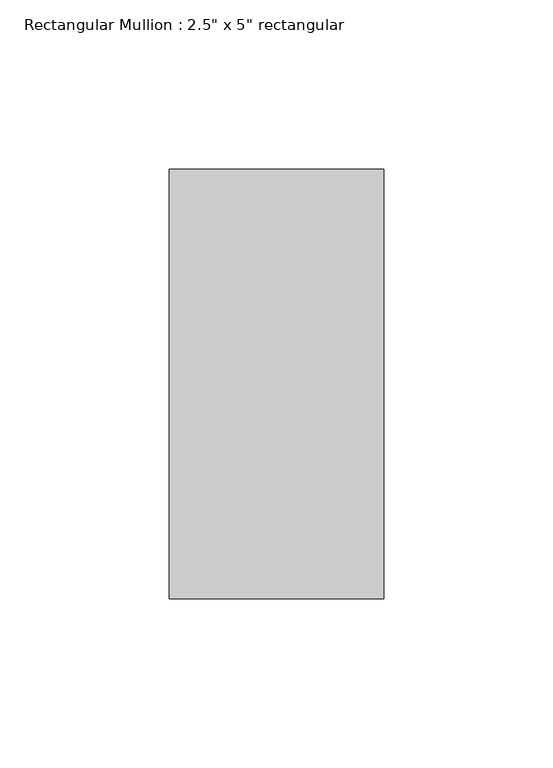
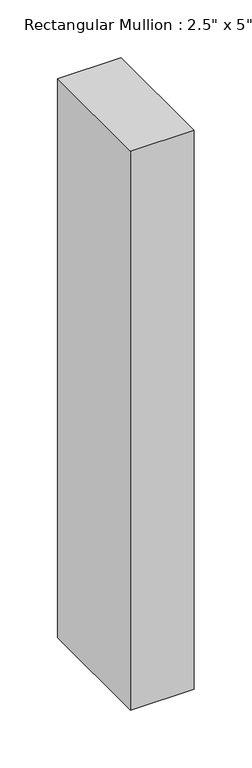
"""IFC4 building model written with IfcOpenShell, lengths in millimetres: member geometry."""

from ifc_helpers import new_model, si_unit, frame, origin, place, context, project, spatial, polyline, outline, extrude, source, transform, mapped, element, save


def member_96ae0c19(model_context):
    return source(origin(), model_context, "Body", "SweptSolid", [
        extrude(outline(polyline([(0.0, 63.5), (0.0, -63.5), (-63.5, -63.5), (-63.5, 63.5), (0.0, 63.5)])), frame((0.0, 0.0, -591.3271638), z_axis=(0.0, 0.0, 1.0), x_axis=(1.0, 0.0, 0.0)), (0.0, 0.0, 1.0), 591.3271638),
    ])


if __name__ == "__main__":
    model = new_model("IFC4")
    model_context = context("Model", 3, world=origin())
    ifc_project = project(units=[si_unit("LENGTHUNIT", "METRE", prefix="MILLI")], contexts=[model_context])
    site = spatial("IfcSite", under=ifc_project)
    building = spatial("IfcBuilding", under=site)
    placement = place(None, origin())
    member_shape = member_96ae0c19(model_context)
    element("IfcMember", 1, ObjectType="Rectangular Mullion : 2.5\" x 5\" rectangular", at=placement, inside=building, context=model_context, shape_type="MappedRepresentation", body=[
        mapped(member_shape, transform((0.0, 0.0, 0.0), x_axis=(1.0, 0.0, 0.0), y_axis=(0.0, 1.0, 0.0), z_axis=(0.0, 0.0, 1.0))),
    ])
    save(model, "model.ifc")

# Revit data of these elements
# Type "Rectangular Mullion : 2.5\" x 5\" rectangular"
#   built-in parameter 1007304 = 0.416667 (stored number, unit not read)
#   built-in parameter 1007301 = 0.104167 (stored number, unit not read)
#   built-in parameter 1007300 = 0.104167 (stored number, unit not read)
# Element 1 (IfcMember, "Rectangular Mullion : 2.5\" x 5\" rectangular")
#   Materials on its faces: "Aluminum"
# Materials
#   "Aluminum": class "Metal", colour RGB 247 247 247, transparency 0, Description = "Aluminum 6061", Cost = 0
